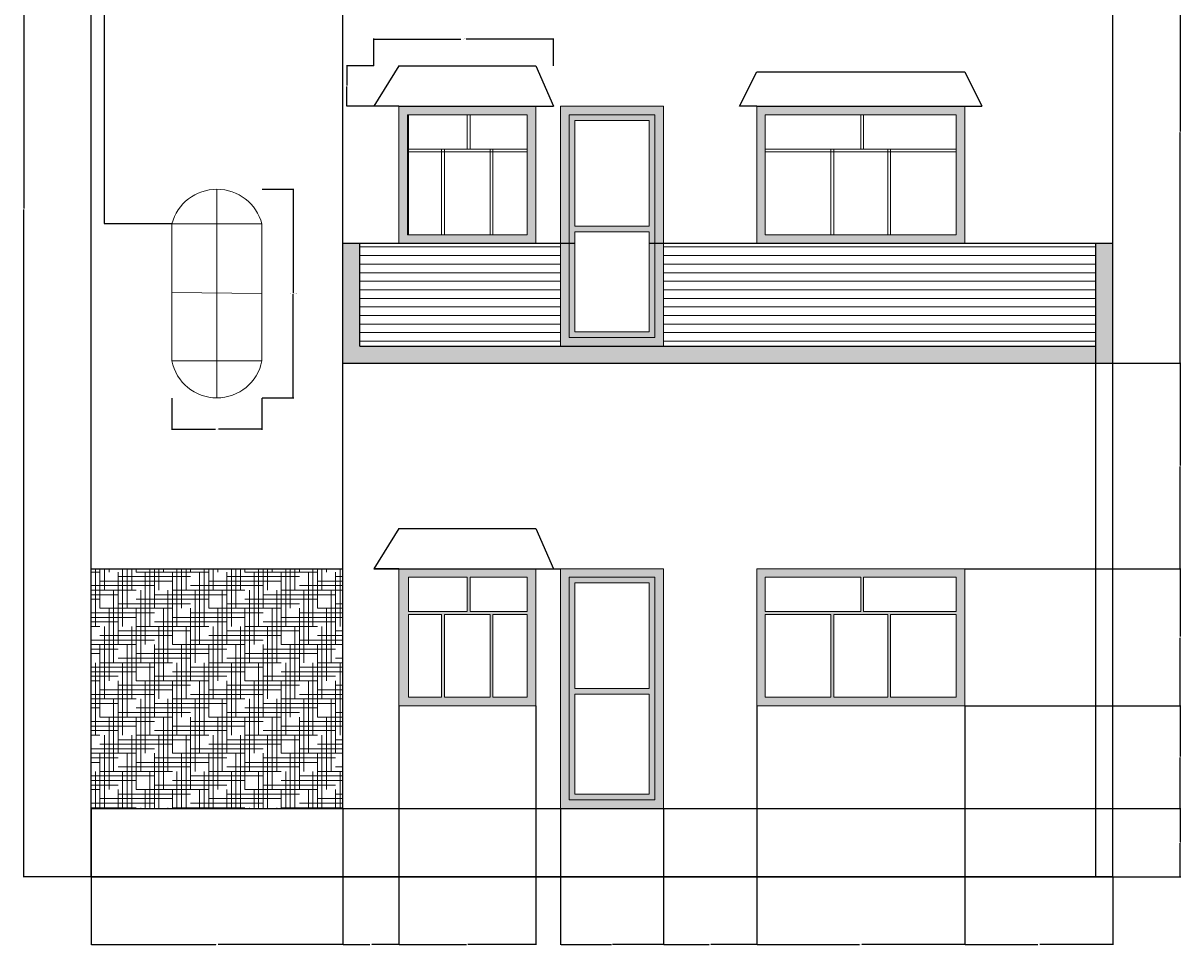
# Model space of a CAD drawing. Units: inches. Extents: x 3504 to 4623, y 2365 to 3357.
# Tile 2 of 5: x 3504 to 3909, y 2841 to 3164. Entities that reach past the tile are written whole.
import ezdxf

# ---------------------------------------------------------------- set-up
doc = ezdxf.new("R2010")
doc.units = ezdxf.units.IN
for name, color, linetype, lineweight in [('A-ANNO-DIMS', 2, 'Continuous', 18), ('A-DOOR', 3, 'Continuous', 18), ('A-ELEV', 7, 'Continuous', 25), ('A-ELEV-PATT', 7, 'Continuous', 13), ('A-FLOR-HRAL', 7, 'Continuous', 25), ('A-FLOR-HRAL-PATT', 252, 'Continuous', 13), ('A-GLAZ', 4, 'Continuous', 18), ('A-ROOF', 7, 'Continuous', 25)]:
    doc.layers.add(name, color=color, linetype=linetype, lineweight=lineweight)
doc.styles.get("Standard").update_dxf_attribs({"font": 'arial.ttf'})
doc.dimstyles.get("Standard").update_dxf_attribs({"dimtxt": 0.18, "dimasz": 0.18, "dimexe": 0.18, "dimexo": 0.0625, "dimgap": 0.09, "dimtad": 0, "dimtih": 1, "dimtoh": 1, "dimdec": 4, "dimzin": 0, "dimdsep": 46, "dimtxsty": 'Standard', "dimcen": 0.09, "dimadec": 0, "dimazin": 0, "dimtfac": 1, "dimtdec": 4, "dimtofl": 0, "dimtmove": 0, "dimatfit": 3, "dimfxl": 1, "dimtolj": 1, "dimtzin": 0, "dimarcsym": 0})

# ---------------------------------------------------------------- blocks, each defined once
blk = doc.blocks.new('WIN-ARCH-END-ELEV')
for p, q in [((15.78, 73.08), (15.78, 0)), ((0, 60.97), (31.56, 60.97)), ((0, 60.97), (0, 12.97)), ((31.56, 12.97), (31.56, 60.97)), ((0, 36.97), (31.56, 36.54)), ((0, 12.97), (31.56, 12.97)), ((0, 12.97), (31.56, 12.97))]:
    blk.add_line(p, q)
for centre, radius, start, end in [((15.78, 56.75), 16.33, 14.9627, 165.0373), ((15.78, 16.08), 16.08, 191.1699, 348.8301)]:
    blk.add_arc(centre, radius, start, end)
blk = doc.blocks.new('WINDOW-HOOD-CAP-48')
for p, q in [((8.73, 14.1), (0, 0)), ((8.73, 14.1), (56.73, 14.1)), ((56.73, 14.1), (62.87, 0))]:
    blk.add_line(p, q)
blk = doc.blocks.new('*D19')
at = {"layer": 'A-ANNO-DIMS', "color": 0, "lineweight": -2, "transparency": 16777216}
for p, q in [((3587.42, 3105.9), (3598.5, 3105.9)), ((3598.32, 3105.72), (3598.32, 3069.54)), ((3598.32, 3032.99), (3598.32, 3069.17)), ((3587.42, 3032.81), (3598.5, 3032.81))]:
    blk.add_line(p, q, dxfattribs=at)
at = {"layer": 'A-ANNO-DIMS', "color": 0, "transparency": 16777216}
for points in [[(3598.29, 3105.72), (3598.35, 3105.72), (3598.32, 3105.9)], [(3598.29, 3032.99), (3598.35, 3032.99), (3598.32, 3032.81)]]:
    blk.add_solid(points, dxfattribs=at)
at = {"layer": 'Defpoints', "color": 0, "transparency": 16777216}
for p in [(3587.36, 3105.9), (3598.32, 3105.9), (3587.36, 3032.81)]:
    blk.add_point(p, dxfattribs=at)
at = {"layer": 'A-ANNO-DIMS', "color": 0, "transparency": 16777216, "insert": (3598.32, 3069.35), "char_height": 0.18, "attachment_point": 5}
blk.add_mtext('\\A1;STAIR WINDOW 73 TYP.', dxfattribs=at)
blk = doc.blocks.new('*D20')
at = {"layer": 'A-ANNO-DIMS', "color": 0, "lineweight": -2, "transparency": 16777216}
for p, q in [((3555.8, 3032.75), (3555.8, 3021.67)), ((3587.36, 3032.75), (3587.36, 3021.67)), ((3555.98, 3021.85), (3571.05, 3021.85)), ((3587.18, 3021.85), (3572.11, 3021.85))]:
    blk.add_line(p, q, dxfattribs=at)
at = {"layer": 'A-ANNO-DIMS', "color": 0, "transparency": 16777216}
for points in [[(3555.98, 3021.88), (3555.98, 3021.82), (3555.8, 3021.85)], [(3587.18, 3021.88), (3587.18, 3021.82), (3587.36, 3021.85)]]:
    blk.add_solid(points, dxfattribs=at)
at = {"layer": 'Defpoints', "color": 0, "transparency": 16777216}
for p in [(3555.8, 3032.81), (3587.36, 3032.81), (3587.36, 3021.85)]:
    blk.add_point(p, dxfattribs=at)
at = {"layer": 'A-ANNO-DIMS', "color": 0, "transparency": 16777216, "insert": (3571.58, 3021.85), "char_height": 0.18, "attachment_point": 5}
blk.add_mtext('\\A1;32 TYP.', dxfattribs=at)
blk = doc.blocks.new('*D21')
at = {"layer": 'A-ANNO-DIMS', "color": 0, "lineweight": -2, "transparency": 16777216}
for p, q in [((3626.58, 3149.15), (3626.58, 3158.69)), ((3626.76, 3158.51), (3657.08, 3158.51)), ((3689.27, 3158.51), (3658.95, 3158.51)), ((3689.45, 3149.15), (3689.45, 3158.69))]:
    blk.add_line(p, q, dxfattribs=at)
at = {"layer": 'A-ANNO-DIMS', "color": 0, "transparency": 16777216}
for points in [[(3626.76, 3158.54), (3626.76, 3158.48), (3626.58, 3158.51)], [(3689.27, 3158.54), (3689.27, 3158.48), (3689.45, 3158.51)]]:
    blk.add_solid(points, dxfattribs=at)
at = {"layer": 'Defpoints', "color": 0, "transparency": 16777216}
for p in [(3689.45, 3158.51), (3626.58, 3149.08), (3689.45, 3149.08)]:
    blk.add_point(p, dxfattribs=at)
at = {"layer": 'A-ANNO-DIMS', "color": 0, "transparency": 16777216, "insert": (3658.01, 3158.51), "char_height": 0.18, "attachment_point": 5}
blk.add_mtext('\\A1;HOOD 63 TYP.', dxfattribs=at)
blk = doc.blocks.new('*D22')
at = {"layer": 'A-ANNO-DIMS', "color": 0, "lineweight": -2, "transparency": 16777216}
for p, q in [((3626.52, 3149.08), (3616.97, 3149.08)), ((3617.15, 3148.9), (3617.15, 3142.21)), ((3617.15, 3135.16), (3617.15, 3141.85)), ((3626.52, 3134.98), (3616.97, 3134.98))]:
    blk.add_line(p, q, dxfattribs=at)
at = {"layer": 'A-ANNO-DIMS', "color": 0, "transparency": 16777216}
for points in [[(3617.12, 3148.9), (3617.18, 3148.9), (3617.15, 3149.08)], [(3617.12, 3135.16), (3617.18, 3135.16), (3617.15, 3134.98)]]:
    blk.add_solid(points, dxfattribs=at)
at = {"layer": 'Defpoints', "color": 0, "transparency": 16777216}
for p in [(3617.15, 3149.08), (3626.58, 3149.08), (3626.58, 3134.98)]:
    blk.add_point(p, dxfattribs=at)
at = {"layer": 'A-ANNO-DIMS', "color": 0, "transparency": 16777216, "insert": (3617.15, 3142.03), "char_height": 0.18, "attachment_point": 5}
blk.add_mtext('\\A1;14 TYP.', dxfattribs=at)
blk = doc.blocks.new('*D48')
at = {"layer": 'A-ANNO-DIMS', "color": 0, "lineweight": -2, "transparency": 16777216}
for p, q in [((3527.5, 2888.92), (3527.5, 2841.2)), ((3615.67, 2888.92), (3615.67, 2841.2)), ((3527.68, 2841.38), (3571.19, 2841.38)), ((3615.49, 2841.38), (3571.98, 2841.38))]:
    blk.add_line(p, q, dxfattribs=at)
at = {"layer": 'A-ANNO-DIMS', "color": 0, "transparency": 16777216}
for points in [[(3527.68, 2841.41), (3527.68, 2841.35), (3527.5, 2841.38)], [(3615.49, 2841.41), (3615.49, 2841.35), (3615.67, 2841.38)]]:
    blk.add_solid(points, dxfattribs=at)
at = {"layer": 'Defpoints', "color": 0, "transparency": 16777216}
for p in [(3527.5, 2888.98), (3615.67, 2888.98), (3615.67, 2841.38)]:
    blk.add_point(p, dxfattribs=at)
at = {"layer": 'A-ANNO-DIMS', "color": 0, "transparency": 16777216, "insert": (3571.58, 2841.38), "char_height": 0.18, "attachment_point": 5}
blk.add_mtext('\\A1;88.17', dxfattribs=at)
blk = doc.blocks.new('*D49')
at = {"layer": 'A-ANNO-DIMS', "color": 0, "lineweight": -2, "transparency": 16777216}
for p, q in [((3635.31, 2924.92), (3635.31, 2841.2)), ((3615.67, 2888.92), (3615.67, 2841.2)), ((3615.85, 2841.38), (3625.1, 2841.38)), ((3635.13, 2841.38), (3625.87, 2841.38))]:
    blk.add_line(p, q, dxfattribs=at)
at = {"layer": 'A-ANNO-DIMS', "color": 0, "transparency": 16777216}
for points in [[(3615.85, 2841.41), (3615.85, 2841.35), (3615.67, 2841.38)], [(3635.13, 2841.41), (3635.13, 2841.35), (3635.31, 2841.38)]]:
    blk.add_solid(points, dxfattribs=at)
at = {"layer": 'Defpoints', "color": 0, "transparency": 16777216}
for p in [(3635.31, 2924.98), (3615.67, 2888.98), (3635.31, 2841.38)]:
    blk.add_point(p, dxfattribs=at)
at = {"layer": 'A-ANNO-DIMS', "color": 0, "transparency": 16777216, "insert": (3625.49, 2841.38), "char_height": 0.18, "attachment_point": 5}
blk.add_mtext('\\A1;19.64', dxfattribs=at)
blk = doc.blocks.new('*D50')
at = {"layer": 'A-ANNO-DIMS', "color": 0, "lineweight": -2, "transparency": 16777216}
for p, q in [((3635.31, 2924.92), (3635.31, 2841.2)), ((3683.31, 2924.92), (3683.31, 2841.2)), ((3635.49, 2841.38), (3659.08, 2841.38)), ((3683.13, 2841.38), (3659.53, 2841.38))]:
    blk.add_line(p, q, dxfattribs=at)
at = {"layer": 'A-ANNO-DIMS', "color": 0, "transparency": 16777216}
for points in [[(3635.49, 2841.41), (3635.49, 2841.35), (3635.31, 2841.38)], [(3683.13, 2841.41), (3683.13, 2841.35), (3683.31, 2841.38)]]:
    blk.add_solid(points, dxfattribs=at)
at = {"layer": 'Defpoints', "color": 0, "transparency": 16777216}
for p in [(3635.31, 2924.98), (3683.31, 2924.98), (3683.31, 2841.38)]:
    blk.add_point(p, dxfattribs=at)
at = {"layer": 'A-ANNO-DIMS', "color": 0, "transparency": 16777216, "insert": (3659.31, 2841.38), "char_height": 0.18, "attachment_point": 5}
blk.add_mtext('\\A1;48', dxfattribs=at)
blk = doc.blocks.new('*D51')
at = {"layer": 'A-ANNO-DIMS', "color": 0, "lineweight": -2, "transparency": 16777216}
for p, q in [((3692, 2888.92), (3692, 2841.2)), ((3728, 2888.92), (3728, 2841.2)), ((3692.18, 2841.38), (3709.78, 2841.38)), ((3727.82, 2841.38), (3710.22, 2841.38))]:
    blk.add_line(p, q, dxfattribs=at)
at = {"layer": 'A-ANNO-DIMS', "color": 0, "transparency": 16777216}
for points in [[(3692.18, 2841.41), (3692.18, 2841.35), (3692, 2841.38)], [(3727.82, 2841.41), (3727.82, 2841.35), (3728, 2841.38)]]:
    blk.add_solid(points, dxfattribs=at)
at = {"layer": 'Defpoints', "color": 0, "transparency": 16777216}
for p in [(3692, 2888.98), (3728, 2888.98), (3728, 2841.38)]:
    blk.add_point(p, dxfattribs=at)
at = {"layer": 'A-ANNO-DIMS', "color": 0, "transparency": 16777216, "insert": (3710, 2841.38), "char_height": 0.18, "attachment_point": 5}
blk.add_mtext('\\A1;36', dxfattribs=at)
blk = doc.blocks.new('*D52')
at = {"layer": 'A-ANNO-DIMS', "color": 0, "lineweight": -2, "transparency": 16777216}
for p, q in [((3760.69, 2924.92), (3760.69, 2841.2)), ((3728, 2888.92), (3728, 2841.2)), ((3728.18, 2841.38), (3744.02, 2841.38)), ((3760.51, 2841.38), (3744.67, 2841.38))]:
    blk.add_line(p, q, dxfattribs=at)
at = {"layer": 'A-ANNO-DIMS', "color": 0, "transparency": 16777216}
for points in [[(3728.18, 2841.41), (3728.18, 2841.35), (3728, 2841.38)], [(3760.51, 2841.41), (3760.51, 2841.35), (3760.69, 2841.38)]]:
    blk.add_solid(points, dxfattribs=at)
at = {"layer": 'Defpoints', "color": 0, "transparency": 16777216}
for p in [(3760.69, 2924.98), (3728, 2888.98), (3760.69, 2841.38)]:
    blk.add_point(p, dxfattribs=at)
at = {"layer": 'A-ANNO-DIMS', "color": 0, "transparency": 16777216, "insert": (3744.35, 2841.38), "char_height": 0.18, "attachment_point": 5}
blk.add_mtext('\\A1;32.7', dxfattribs=at)
blk = doc.blocks.new('*D53')
at = {"layer": 'A-ANNO-DIMS', "color": 0, "lineweight": -2, "transparency": 16777216}
for p, q in [((3760.69, 2924.92), (3760.69, 2841.2)), ((3833.61, 2924.92), (3833.61, 2841.2)), ((3760.87, 2841.38), (3796.76, 2841.38)), ((3833.43, 2841.38), (3797.55, 2841.38))]:
    blk.add_line(p, q, dxfattribs=at)
at = {"layer": 'A-ANNO-DIMS', "color": 0, "transparency": 16777216}
for points in [[(3760.87, 2841.41), (3760.87, 2841.35), (3760.69, 2841.38)], [(3833.43, 2841.41), (3833.43, 2841.35), (3833.61, 2841.38)]]:
    blk.add_solid(points, dxfattribs=at)
at = {"layer": 'Defpoints', "color": 0, "transparency": 16777216}
for p in [(3760.69, 2924.98), (3833.61, 2924.98), (3833.61, 2841.38)]:
    blk.add_point(p, dxfattribs=at)
at = {"layer": 'A-ANNO-DIMS', "color": 0, "transparency": 16777216, "insert": (3797.15, 2841.38), "char_height": 0.18, "attachment_point": 5}
blk.add_mtext('\\A1;72.92', dxfattribs=at)
blk = doc.blocks.new('*D54')
at = {"layer": 'A-ANNO-DIMS', "color": 0, "lineweight": -2, "transparency": 16777216}
for p, q in [((3833.61, 2924.92), (3833.61, 2841.2)), ((3885.5, 2864.92), (3885.5, 2841.2)), ((3833.79, 2841.38), (3859.16, 2841.38)), ((3885.32, 2841.38), (3859.95, 2841.38))]:
    blk.add_line(p, q, dxfattribs=at)
at = {"layer": 'A-ANNO-DIMS', "color": 0, "transparency": 16777216}
for points in [[(3833.79, 2841.41), (3833.79, 2841.35), (3833.61, 2841.38)], [(3885.32, 2841.41), (3885.32, 2841.35), (3885.5, 2841.38)]]:
    blk.add_solid(points, dxfattribs=at)
at = {"layer": 'Defpoints', "color": 0, "transparency": 16777216}
for p in [(3833.61, 2924.98), (3885.5, 2864.98), (3885.5, 2841.38)]:
    blk.add_point(p, dxfattribs=at)
at = {"layer": 'A-ANNO-DIMS', "color": 0, "transparency": 16777216, "insert": (3859.55, 2841.38), "char_height": 0.18, "attachment_point": 5}
blk.add_mtext('\\A1;51.88', dxfattribs=at)
blk = doc.blocks.new('*D55')
at = {"layer": 'A-ANNO-DIMS', "color": 0, "lineweight": -2, "transparency": 16777216}
for p, q in [((3885.56, 2888.98), (3909.28, 2888.98)), ((3909.1, 2888.8), (3909.1, 2877.16)), ((3909.1, 2865.16), (3909.1, 2876.8)), ((3885.56, 2864.98), (3909.28, 2864.98))]:
    blk.add_line(p, q, dxfattribs=at)
at = {"layer": 'A-ANNO-DIMS', "color": 0, "transparency": 16777216}
for points in [[(3909.07, 2888.8), (3909.13, 2888.8), (3909.1, 2888.98)], [(3909.07, 2865.16), (3909.13, 2865.16), (3909.1, 2864.98)]]:
    blk.add_solid(points, dxfattribs=at)
at = {"layer": 'Defpoints', "color": 0, "transparency": 16777216}
for p in [(3885.5, 2888.98), (3909.1, 2888.98), (3885.5, 2864.98)]:
    blk.add_point(p, dxfattribs=at)
at = {"layer": 'A-ANNO-DIMS', "color": 0, "transparency": 16777216, "insert": (3909.1, 2876.98), "char_height": 0.18, "attachment_point": 5}
blk.add_mtext('\\A1;24', dxfattribs=at)
blk = doc.blocks.new('*D56')
at = {"layer": 'A-ANNO-DIMS', "color": 0, "lineweight": -2, "transparency": 16777216}
for p, q in [((3833.68, 2924.98), (3909.28, 2924.98)), ((3909.1, 2924.8), (3909.1, 2907.17)), ((3909.1, 2889.16), (3909.1, 2906.8)), ((3885.56, 2888.98), (3909.28, 2888.98))]:
    blk.add_line(p, q, dxfattribs=at)
at = {"layer": 'A-ANNO-DIMS', "color": 0, "transparency": 16777216}
for points in [[(3909.07, 2924.8), (3909.13, 2924.8), (3909.1, 2924.98)], [(3909.07, 2889.16), (3909.13, 2889.16), (3909.1, 2888.98)]]:
    blk.add_solid(points, dxfattribs=at)
at = {"layer": 'Defpoints', "color": 0, "transparency": 16777216}
for p in [(3833.61, 2924.98), (3909.1, 2924.98), (3885.5, 2888.98)]:
    blk.add_point(p, dxfattribs=at)
at = {"layer": 'A-ANNO-DIMS', "color": 0, "transparency": 16777216, "insert": (3909.1, 2906.98), "char_height": 0.18, "attachment_point": 5}
blk.add_mtext('\\A1;36', dxfattribs=at)
blk = doc.blocks.new('*D57')
at = {"layer": 'A-ANNO-DIMS', "color": 0, "lineweight": -2, "transparency": 16777216}
for p, q in [((3833.68, 2972.98), (3909.28, 2972.98)), ((3909.1, 2972.8), (3909.1, 2949.17)), ((3909.1, 2925.16), (3909.1, 2948.8)), ((3833.68, 2924.98), (3909.28, 2924.98))]:
    blk.add_line(p, q, dxfattribs=at)
at = {"layer": 'A-ANNO-DIMS', "color": 0, "transparency": 16777216}
for points in [[(3909.07, 2972.8), (3909.13, 2972.8), (3909.1, 2972.98)], [(3909.07, 2925.16), (3909.13, 2925.16), (3909.1, 2924.98)]]:
    blk.add_solid(points, dxfattribs=at)
at = {"layer": 'Defpoints', "color": 0, "transparency": 16777216}
for p in [(3833.61, 2972.98), (3909.1, 2972.98), (3833.61, 2924.98)]:
    blk.add_point(p, dxfattribs=at)
at = {"layer": 'A-ANNO-DIMS', "color": 0, "transparency": 16777216, "insert": (3909.1, 2948.98), "char_height": 0.18, "attachment_point": 5}
blk.add_mtext('\\A1;48', dxfattribs=at)
blk = doc.blocks.new('*D58')
at = {"layer": 'A-ANNO-DIMS', "color": 0, "lineweight": -2, "transparency": 16777216}
for p, q in [((3885.56, 3044.98), (3909.28, 3044.98)), ((3909.1, 3044.8), (3909.1, 3009.16)), ((3909.1, 2973.16), (3909.1, 3008.8)), ((3833.68, 2972.98), (3909.28, 2972.98))]:
    blk.add_line(p, q, dxfattribs=at)
at = {"layer": 'A-ANNO-DIMS', "color": 0, "transparency": 16777216}
for points in [[(3909.07, 3044.8), (3909.13, 3044.8), (3909.1, 3044.98)], [(3909.07, 2973.16), (3909.13, 2973.16), (3909.1, 2972.98)]]:
    blk.add_solid(points, dxfattribs=at)
at = {"layer": 'Defpoints', "color": 0, "transparency": 16777216}
for p in [(3885.5, 3044.98), (3909.1, 3044.98), (3833.61, 2972.98)]:
    blk.add_point(p, dxfattribs=at)
at = {"layer": 'A-ANNO-DIMS', "color": 0, "transparency": 16777216, "insert": (3909.1, 3008.98), "char_height": 0.18, "attachment_point": 5}
blk.add_mtext('\\A1;72', dxfattribs=at)
blk = doc.blocks.new('*D59')
at = {"layer": 'A-ANNO-DIMS', "color": 0, "lineweight": -2, "transparency": 16777216}
for p, q in [((3885.56, 3206.98), (3909.28, 3206.98)), ((3909.1, 3206.8), (3909.1, 3126.17)), ((3909.1, 3045.16), (3909.1, 3125.8)), ((3885.56, 3044.98), (3909.28, 3044.98))]:
    blk.add_line(p, q, dxfattribs=at)
at = {"layer": 'A-ANNO-DIMS', "color": 0, "transparency": 16777216}
for points in [[(3909.07, 3206.8), (3909.13, 3206.8), (3909.1, 3206.98)], [(3909.07, 3045.16), (3909.13, 3045.16), (3909.1, 3044.98)]]:
    blk.add_solid(points, dxfattribs=at)
at = {"layer": 'Defpoints', "color": 0, "transparency": 16777216}
for p in [(3885.5, 3206.98), (3909.1, 3206.98), (3885.5, 3044.98)]:
    blk.add_point(p, dxfattribs=at)
at = {"layer": 'A-ANNO-DIMS', "color": 0, "transparency": 16777216, "insert": (3909.1, 3125.98), "char_height": 0.18, "attachment_point": 5}
blk.add_mtext('\\A1;162', dxfattribs=at)
blk = doc.blocks.new('*D61')
at = {"layer": 'A-ANNO-DIMS', "color": 0, "lineweight": -2, "transparency": 16777216}
for p, q in [((3555.74, 3260.98), (3532.02, 3260.98)), ((3532.2, 3260.8), (3532.2, 3177.56)), ((3532.2, 3093.96), (3532.2, 3177.2)), ((3555.74, 3093.78), (3532.02, 3093.78))]:
    blk.add_line(p, q, dxfattribs=at)
at = {"layer": 'A-ANNO-DIMS', "color": 0, "transparency": 16777216}
for points in [[(3532.17, 3260.8), (3532.23, 3260.8), (3532.2, 3260.98)], [(3532.17, 3093.96), (3532.23, 3093.96), (3532.2, 3093.78)]]:
    blk.add_solid(points, dxfattribs=at)
at = {"layer": 'Defpoints', "color": 0, "transparency": 16777216}
for p in [(3532.2, 3260.98), (3555.8, 3260.98), (3555.8, 3093.78)]:
    blk.add_point(p, dxfattribs=at)
at = {"layer": 'A-ANNO-DIMS', "color": 0, "transparency": 16777216, "insert": (3532.2, 3177.38), "char_height": 0.18, "attachment_point": 5}
blk.add_mtext('\\A1;167.2', dxfattribs=at)
blk = doc.blocks.new('*D63')
at = {"layer": 'A-ANNO-DIMS', "color": 0, "lineweight": -2, "transparency": 16777216}
for p, q in [((3527.43, 3332.98), (3503.72, 3332.98)), ((3503.9, 3332.8), (3503.9, 3099.17)), ((3503.9, 2865.16), (3503.9, 3098.8)), ((3527.43, 2864.98), (3503.72, 2864.98))]:
    blk.add_line(p, q, dxfattribs=at)
at = {"layer": 'A-ANNO-DIMS', "color": 0, "transparency": 16777216}
for points in [[(3503.87, 3332.8), (3503.93, 3332.8), (3503.9, 3332.98)], [(3503.87, 2865.16), (3503.93, 2865.16), (3503.9, 2864.98)]]:
    blk.add_solid(points, dxfattribs=at)
at = {"layer": 'Defpoints', "color": 0, "transparency": 16777216}
for p in [(3503.9, 3332.98), (3527.5, 3332.98), (3527.5, 2864.98)]:
    blk.add_point(p, dxfattribs=at)
at = {"layer": 'A-ANNO-DIMS', "color": 0, "transparency": 16777216, "insert": (3503.9, 3098.98), "char_height": 0.18, "attachment_point": 5}
blk.add_mtext('\\A1;468', dxfattribs=at)

msp = doc.modelspace()

# ---------------------------------------------------------------- hatches: boundary and pattern name
at = {"layer": 'A-ELEV-PATT'}
h = msp.add_hatch(color=256, dxfattribs=at)
h.dxf.hatch_style = 1
h.paths.add_polyline_path([(3683.3055, 3134.9837), (3635.3055, 3134.9837), (3635.3055, 3086.9837), (3683.3055, 3086.9837)])
h.paths.add_polyline_path([(3680.3055, 3131.9837), (3680.3055, 3089.9837), (3638.3055, 3089.9837), (3638.3055, 3131.9837)], flags=16)
h.paths.add_polyline_path([(3668.3055, 3119.9837), (3668.3055, 3118.9837), (3638.6868, 3118.9837), (3638.6868, 3119.9837)], flags=0)
h.paths.add_polyline_path([(3651.3055, 3118.9837), (3650.3055, 3118.9837), (3650.3055, 3089.9837), (3651.3055, 3089.9837)], flags=0)
h.paths.add_polyline_path([(3668.3055, 3118.9837), (3667.3055, 3118.9837), (3667.3055, 3089.9837), (3668.3055, 3089.9837)], flags=0)
h.paths.add_polyline_path([(3724.9963, 3131.9837), (3694.9963, 3131.9837), (3694.9963, 3053.9837), (3724.9963, 3053.9837)], flags=0)
h.paths.add_polyline_path([(3696.9963, 3129.9837), (3722.9963, 3129.9837), (3722.9963, 3092.9837), (3696.9963, 3092.9837)], flags=0)
h.paths.add_polyline_path([(3696.9963, 3090.9837), (3722.9963, 3090.9837), (3722.9963, 3055.9837), (3696.9963, 3055.9837)], flags=0)
h.paths.add_polyline_path([(3727.9963, 3134.9837), (3691.9963, 3134.9837), (3691.9963, 3050.9837), (3727.9963, 3050.9837)])
h.paths.add_polyline_path([(3694.9963, 3131.9837), (3724.9963, 3131.9837), (3724.9963, 3053.9837), (3694.9963, 3053.9837)], flags=16)
h.paths.add_polyline_path([(3833.6131, 3134.9837), (3760.6941, 3134.9837), (3760.6941, 3086.9837), (3833.6131, 3086.9837)])
h.paths.add_polyline_path([(3763.6941, 3131.9837), (3830.6131, 3131.9837), (3830.6131, 3089.9837), (3763.6941, 3089.9837)], flags=16)
h.paths.add_polyline_path([(3807.6131, 3119.9837), (3807.6131, 3118.9837), (3786.6941, 3118.9837), (3786.6941, 3119.9837)], flags=0)
h.paths.add_polyline_path([(3680.3055, 3119.9837), (3668.3055, 3119.9837), (3668.3055, 3118.9837), (3680.3055, 3118.9837)], flags=0)
h.paths.add_polyline_path([(3660.3055, 3131.9837), (3659.3055, 3131.9837), (3659.3055, 3119.9837), (3660.3055, 3119.9837)], flags=0)
h.paths.add_polyline_path([(3787.6941, 3118.9837), (3786.6941, 3118.9837), (3786.6941, 3089.9837), (3787.6941, 3089.9837)], flags=0)
h.paths.add_polyline_path([(3807.6131, 3118.9837), (3806.6131, 3118.9837), (3806.6131, 3089.9837), (3807.6131, 3089.9837)], flags=0)
h.paths.add_polyline_path([(3786.6941, 3119.9837), (3763.6941, 3119.9837), (3763.6941, 3118.9837), (3786.6941, 3118.9837)], flags=0)
h.paths.add_polyline_path([(3787.6941, 3119.9837), (3786.6941, 3119.9837), (3786.6941, 3118.9837), (3787.6941, 3118.9837)], flags=0)
h.paths.add_polyline_path([(3807.6131, 3119.9837), (3806.6131, 3119.9837), (3806.6131, 3118.9837), (3807.6131, 3118.9837)], flags=0)
h.paths.add_polyline_path([(3798.1536, 3131.9837), (3797.1536, 3131.9837), (3797.1536, 3119.9837), (3798.1536, 3119.9837)], flags=0)
h.paths.add_polyline_path([(3830.6131, 3119.9837), (3807.6131, 3119.9837), (3807.6131, 3118.9837), (3830.6131, 3118.9837)], flags=0)
h = msp.add_hatch(color=256, dxfattribs=at)
h.dxf.hatch_style = 1
h.paths.add_polyline_path([(3724.9963, 3131.9837), (3694.9963, 3131.9837), (3694.9963, 3053.9837), (3724.9963, 3053.9837)])
h.paths.add_polyline_path([(3696.9963, 3092.9837), (3696.9963, 3129.9837), (3722.9963, 3129.9837), (3722.9963, 3092.9837)], flags=16)
h.paths.add_polyline_path([(3722.9963, 3090.9837), (3722.9963, 3055.9837), (3696.9963, 3055.9837), (3696.9963, 3090.9837)], flags=16)
h = msp.add_hatch(color=256, dxfattribs=at)
h.dxf.hatch_style = 1
h.paths.add_polyline_path([(3885.4963, 3086.9837), (3879.4963, 3086.9837), (3879.4963, 3050.9837), (3621.6665, 3050.9837), (3621.6665, 3086.9837), (3615.6665, 3086.9837), (3615.6665, 3044.9837), (3885.4963, 3044.9837)])
h = msp.add_hatch(dxfattribs=at)
h.set_pattern_fill('HOUND', color=256)
h.paths.add_polyline_path([(3527.4963, 2972.9837), (3527.4963, 2888.9837), (3615.6665, 2888.9837), (3615.6665, 2972.9837)])
h = msp.add_hatch(color=256, dxfattribs=at)
h.dxf.hatch_style = 1
h.paths.add_polyline_path([(3683.3055, 2972.9837), (3635.3055, 2972.9837), (3635.3055, 2924.9837), (3683.3055, 2924.9837)])
h.paths.add_polyline_path([(3638.6868, 2956.9837), (3650.3055, 2956.9837), (3650.3055, 2927.9837), (3638.6868, 2927.9837)], flags=16)
h.paths.add_polyline_path([(3651.3055, 2956.9837), (3667.3055, 2956.9837), (3667.3055, 2927.9837), (3651.3055, 2927.9837)], flags=16)
h.paths.add_polyline_path([(3638.6868, 2957.9837), (3638.6868, 2969.9837), (3659.3055, 2969.9837), (3659.3055, 2957.9837)], flags=16)
h.paths.add_polyline_path([(3660.3055, 2957.9837), (3660.3055, 2969.9837), (3680.3055, 2969.9837), (3680.3055, 2957.9837)], flags=16)
h.paths.add_polyline_path([(3668.3055, 2956.9837), (3680.3055, 2956.9837), (3680.3055, 2927.9837), (3668.3055, 2927.9837)], flags=16)
h = msp.add_hatch(color=256, dxfattribs=at)
h.dxf.hatch_style = 1
h.paths.add_polyline_path([(3724.9963, 2969.9837), (3694.9963, 2969.9837), (3694.9963, 2891.9837), (3724.9963, 2891.9837)], flags=0)
h.paths.add_polyline_path([(3696.9963, 2967.9837), (3722.9963, 2967.9837), (3722.9963, 2930.9837), (3696.9963, 2930.9837)], flags=0)
h.paths.add_polyline_path([(3696.9963, 2928.9837), (3722.9963, 2928.9837), (3722.9963, 2893.9837), (3696.9963, 2893.9837)], flags=0)
h.paths.add_polyline_path([(3727.9963, 2972.9837), (3691.9963, 2972.9837), (3691.9963, 2888.9837), (3727.9963, 2888.9837)])
h.paths.add_polyline_path([(3694.9963, 2969.9837), (3724.9963, 2969.9837), (3724.9963, 2891.9837), (3694.9963, 2891.9837)], flags=16)
h = msp.add_hatch(color=256, dxfattribs=at)
h.dxf.hatch_style = 1
h.paths.add_polyline_path([(3724.9963, 2969.9837), (3694.9963, 2969.9837), (3694.9963, 2891.9837), (3724.9963, 2891.9837)])
h.paths.add_polyline_path([(3696.9963, 2930.9837), (3696.9963, 2967.9837), (3722.9963, 2967.9837), (3722.9963, 2930.9837)], flags=16)
h.paths.add_polyline_path([(3722.9963, 2928.9837), (3722.9963, 2893.9837), (3696.9963, 2893.9837), (3696.9963, 2928.9837)], flags=16)
h = msp.add_hatch(color=256, dxfattribs=at)
h.dxf.hatch_style = 1
h.paths.add_polyline_path([(3833.6131, 2972.9837), (3760.6941, 2972.9837), (3760.6941, 2924.9837), (3833.6131, 2924.9837)])
h.paths.add_polyline_path([(3797.1536, 2957.9837), (3763.6941, 2957.9837), (3763.6941, 2969.9837), (3797.1536, 2969.9837)], flags=16)
h.paths.add_polyline_path([(3798.1536, 2969.9837), (3830.6131, 2969.9837), (3830.6131, 2957.9837), (3798.1536, 2957.9837)], flags=16)
h.paths.add_polyline_path([(3806.6131, 2956.9837), (3806.6131, 2927.9837), (3787.6941, 2927.9837), (3787.6941, 2956.9837)], flags=16)
h.paths.add_polyline_path([(3807.6131, 2956.9837), (3830.6131, 2956.9837), (3830.6131, 2927.9837), (3807.6131, 2927.9837)], flags=16)
h.paths.add_polyline_path([(3786.6941, 2956.9837), (3786.6941, 2927.9837), (3763.6941, 2927.9837), (3763.6941, 2956.9837)], flags=16)
at = {"layer": 'A-FLOR-HRAL-PATT'}
h = msp.add_hatch(dxfattribs=at)
h.set_pattern_fill('ANSI31', color=256, scale=0.944475, angle=-45, style=0)
h.paths.add_polyline_path([(3621.6665, 3050.9837), (3691.9963, 3050.9837), (3691.9963, 3086.9837), (3621.6665, 3086.9837)])
h = msp.add_hatch(dxfattribs=at)
h.set_pattern_fill('ANSI31', color=256, scale=0.944475, angle=-45, style=0)
h.paths.add_polyline_path([(3727.9963, 3050.9837), (3879.4963, 3050.9837), (3879.4963, 3086.9837), (3727.9963, 3086.9837)])

# ---------------------------------------------------------------- linework, layer by layer
at = {"layer": 'A-DOOR'}
for p, q in [((3691.9963, 3086.9837), (3691.9963, 3134.9837)), ((3691.9963, 3134.9837), (3727.9963, 3134.9837)), ((3691.9963, 3050.9837), (3691.9963, 3134.9837)), ((3727.9963, 3086.9837), (3727.9963, 3134.9837)), ((3727.9963, 3050.9837), (3727.9963, 3134.9837)), ((3709.9963, 3092.9837), (3696.9963, 3092.9837)), ((3696.9963, 3092.9837), (3722.9963, 3092.9837)), ((3696.9963, 3090.9837), (3722.9963, 3090.9837)), ((3691.9963, 2888.9837), (3691.9963, 2972.9837)), ((3727.9963, 2888.9837), (3727.9963, 2972.9837)), ((3709.9963, 2930.9837), (3696.9963, 2930.9837)), ((3696.9963, 2930.9837), (3722.9963, 2930.9837)), ((3696.9963, 2928.9837), (3722.9963, 2928.9837))]:
    msp.add_line(p, q, dxfattribs=at)
for points in [[(3691.9963, 3050.9837), (3727.9963, 3050.9837), (3727.9963, 3134.9837), (3691.9963, 3134.9837)], [(3691.9963, 3050.9837), (3727.9963, 3050.9837), (3727.9963, 3134.9837), (3691.9963, 3134.9837)], [(3694.9963, 3053.9837), (3724.9963, 3053.9837), (3724.9963, 3131.9837), (3694.9963, 3131.9837)], [(3691.9963, 2888.9837), (3727.9963, 2888.9837), (3727.9963, 2972.9837), (3691.9963, 2972.9837)], [(3694.9963, 2891.9837), (3724.9963, 2891.9837), (3724.9963, 2969.9837), (3694.9963, 2969.9837)]]:
    msp.add_lwpolyline(points, close=True, dxfattribs=at)
for points in [[(3722.9963, 3092.9837), (3722.9963, 3129.9837), (3696.9963, 3129.9837), (3696.9963, 3092.9837)], [(3696.9963, 3090.9837), (3696.9963, 3055.9837), (3722.9963, 3055.9837), (3722.9963, 3090.9837)], [(3722.9963, 2930.9837), (3722.9963, 2967.9837), (3696.9963, 2967.9837), (3696.9963, 2930.9837)], [(3696.9963, 2928.9837), (3696.9963, 2893.9837), (3722.9963, 2893.9837), (3722.9963, 2928.9837)]]:
    msp.add_lwpolyline(points, dxfattribs=at)
at = {"layer": 'A-ELEV'}
for p, q in [((3527.4963, 2864.9837), (3527.4963, 3332.9837)), ((3615.6665, 2888.9837), (3615.6665, 3332.9837)), ((3885.4963, 2864.9837), (3885.4963, 3254.9837)), ((3879.4963, 2864.9837), (3879.4963, 3086.9837)), ((3527.4963, 2972.9837), (3615.6665, 2972.9837)), ((3527.4963, 2888.9837), (3691.9963, 2888.9837)), ((3691.9963, 2888.9837), (3885.4963, 2888.9837)), ((3527.4963, 2864.9837), (3885.4963, 2864.9837)), ((3885.4963, 2864.9837), (3527.4963, 2864.9837)), ((3885.4963, 2864.9837), (3527.4963, 2864.9837))]:
    msp.add_line(p, q, dxfattribs=at)
at = {"layer": 'A-FLOR-HRAL'}
for p, q in [((3615.6665, 3086.9837), (3696.9963, 3086.9837)), ((3621.6665, 3050.9837), (3621.6665, 3086.9837)), ((3722.9963, 3086.9837), (3885.4963, 3086.9837)), ((3879.4963, 3050.9837), (3879.4963, 3086.9837)), ((3621.6665, 3050.9837), (3879.4963, 3050.9837)), ((3615.6665, 3044.9837), (3885.4963, 3044.9837))]:
    msp.add_line(p, q, dxfattribs=at)
at = {"layer": 'A-GLAZ'}
for p, q in [((3635.3055, 3086.9837), (3635.3055, 3134.9837)), ((3635.3055, 3134.9837), (3683.3055, 3134.9837)), ((3635.3055, 3086.9837), (3635.3055, 3134.9837)), ((3635.3055, 3134.9837), (3683.3055, 3134.9837)), ((3638.3055, 3089.9837), (3638.3055, 3131.9837)), ((3638.3055, 3131.9837), (3680.3055, 3131.9837)), ((3638.6868, 3089.9837), (3638.6868, 3131.9837)), ((3659.3055, 3119.9837), (3659.3055, 3131.9837)), ((3660.3055, 3119.9837), (3660.3055, 3131.9837)), ((3680.3055, 3089.9837), (3680.3055, 3131.9837)), ((3683.3055, 3086.9837), (3683.3055, 3134.9837)), ((3683.3055, 3086.9837), (3683.3055, 3134.9837)), ((3760.6941, 3086.9837), (3760.6941, 3134.9837)), ((3760.6941, 3134.9837), (3833.6131, 3134.9837)), ((3760.6941, 3086.9837), (3760.6941, 3134.9837)), ((3833.6131, 3134.9837), (3760.6941, 3134.9837)), ((3760.6941, 3134.9837), (3760.6941, 3086.9837)), ((3830.6131, 3131.9837), (3763.6941, 3131.9837)), ((3763.6941, 3131.9837), (3763.6941, 3089.9837)), ((3797.1536, 3119.9837), (3797.1536, 3131.9837)), ((3798.1536, 3119.9837), (3798.1536, 3131.9837)), ((3830.6131, 3089.9837), (3830.6131, 3131.9837)), ((3833.6131, 3086.9837), (3833.6131, 3134.9837)), ((3833.6131, 3086.9837), (3833.6131, 3134.9837)), ((3833.6131, 3086.9837), (3833.6131, 3134.9837)), ((3638.3055, 3119.9837), (3680.3055, 3119.9837)), ((3650.3055, 3089.9837), (3650.3055, 3119.9837)), ((3651.3055, 3089.9837), (3651.3055, 3119.9837)), ((3667.3055, 3089.9837), (3667.3055, 3119.9837)), ((3668.3055, 3089.9837), (3668.3055, 3119.9837)), ((3830.6131, 3119.9837), (3763.6941, 3119.9837)), ((3786.6941, 3119.9837), (3786.6941, 3089.9837)), ((3787.6941, 3119.9837), (3787.6941, 3089.9837)), ((3806.6131, 3089.9837), (3806.6131, 3119.9837)), ((3807.6131, 3089.9837), (3807.6131, 3119.9837)), ((3638.3055, 3118.9837), (3680.3055, 3118.9837)), ((3830.6131, 3118.9837), (3763.6941, 3118.9837)), ((3635.3055, 3086.9837), (3683.3055, 3086.9837)), ((3635.3055, 3086.9837), (3683.3055, 3086.9837)), ((3638.3055, 3089.9837), (3680.3055, 3089.9837)), ((3760.6941, 3086.9837), (3833.6131, 3086.9837)), ((3760.6941, 3086.9837), (3833.6131, 3086.9837)), ((3760.6941, 3086.9837), (3833.6131, 3086.9837)), ((3833.6131, 3086.9837), (3760.6941, 3086.9837)), ((3760.6941, 3086.9837), (3760.6941, 3086.9837)), ((3760.6941, 3086.9837), (3833.6131, 3086.9837)), ((3763.6941, 3089.9837), (3830.6131, 3089.9837)), ((3833.6131, 3086.9837), (3833.6131, 3086.9837)), ((3635.3055, 2972.9837), (3683.3055, 2972.9837)), ((3635.3055, 2924.9837), (3635.3055, 2972.9837)), ((3638.6868, 2969.9837), (3659.3055, 2969.9837)), ((3638.6868, 2957.9837), (3638.6868, 2969.9837)), ((3659.3055, 2957.9837), (3659.3055, 2969.9837)), ((3660.3055, 2957.9837), (3660.3055, 2969.9837)), ((3660.3055, 2969.9837), (3680.3055, 2969.9837)), ((3680.3055, 2957.9837), (3680.3055, 2969.9837)), ((3683.3055, 2924.9837), (3683.3055, 2972.9837)), ((3760.6941, 2924.9837), (3760.6941, 2972.9837)), ((3833.6131, 2972.9837), (3760.6941, 2972.9837)), ((3760.6941, 2972.9837), (3760.6941, 2924.9837)), ((3763.6941, 2969.9837), (3763.6941, 2957.9837)), ((3797.1536, 2969.9837), (3763.6941, 2969.9837)), ((3797.1536, 2957.9837), (3797.1536, 2969.9837)), ((3830.6131, 2969.9837), (3798.1536, 2969.9837)), ((3798.1536, 2957.9837), (3798.1536, 2969.9837)), ((3830.6131, 2957.9837), (3830.6131, 2969.9837)), ((3833.6131, 2924.9837), (3833.6131, 2972.9837)), ((3833.6131, 2924.9837), (3833.6131, 2972.9837)), ((3638.6868, 2957.9837), (3659.3055, 2957.9837)), ((3638.6868, 2927.9837), (3638.6868, 2956.9837)), ((3638.6868, 2956.9837), (3650.3055, 2956.9837)), ((3650.3055, 2927.9837), (3650.3055, 2956.9837)), ((3651.3055, 2927.9837), (3651.3055, 2956.9837)), ((3651.3055, 2956.9837), (3667.3055, 2956.9837)), ((3660.3055, 2957.9837), (3680.3055, 2957.9837)), ((3667.3055, 2927.9837), (3667.3055, 2956.9837)), ((3668.3055, 2927.9837), (3668.3055, 2956.9837)), ((3668.3055, 2956.9837), (3680.3055, 2956.9837)), ((3680.3055, 2927.9837), (3680.3055, 2956.9837)), ((3797.1536, 2957.9837), (3763.6941, 2957.9837)), ((3786.6941, 2956.9837), (3763.6941, 2956.9837)), ((3763.6941, 2956.9837), (3763.6941, 2927.9837)), ((3786.6941, 2956.9837), (3786.6941, 2927.9837)), ((3787.6941, 2956.9837), (3787.6941, 2927.9837)), ((3806.6131, 2956.9837), (3787.6941, 2956.9837)), ((3830.6131, 2957.9837), (3798.1536, 2957.9837)), ((3806.6131, 2927.9837), (3806.6131, 2956.9837)), ((3807.6131, 2927.9837), (3807.6131, 2956.9837)), ((3830.6131, 2956.9837), (3807.6131, 2956.9837)), ((3830.6131, 2927.9837), (3830.6131, 2956.9837)), ((3635.3055, 2924.9837), (3683.3055, 2924.9837)), ((3638.6868, 2927.9837), (3650.3055, 2927.9837)), ((3651.3055, 2927.9837), (3667.3055, 2927.9837)), ((3668.3055, 2927.9837), (3680.3055, 2927.9837)), ((3760.6941, 2924.9837), (3833.6131, 2924.9837)), ((3760.6941, 2924.9837), (3833.6131, 2924.9837)), ((3833.6131, 2924.9837), (3760.6941, 2924.9837)), ((3760.6941, 2924.9837), (3760.6941, 2924.9837)), ((3760.6941, 2924.9837), (3833.6131, 2924.9837)), ((3763.6941, 2927.9837), (3786.6941, 2927.9837)), ((3787.6941, 2927.9837), (3806.6131, 2927.9837)), ((3807.6131, 2927.9837), (3830.6131, 2927.9837)), ((3833.6131, 2924.9837), (3833.6131, 2924.9837))]:
    msp.add_line(p, q, dxfattribs=at)
for points in [[(3635.3055, 3086.9837), (3683.3055, 3086.9837), (3683.3055, 3134.9837), (3635.3055, 3134.9837)], [(3760.6941, 3086.9837), (3833.6131, 3086.9837), (3833.6131, 3134.9837), (3760.6941, 3134.9837)]]:
    msp.add_lwpolyline(points, close=True, dxfattribs=at)
at = {"layer": 'A-ROOF'}
for p, q in [((3754.6941, 3134.9837), (3760.6941, 3146.9837)), ((3760.6941, 3146.9837), (3833.6131, 3146.9837)), ((3833.6131, 3146.9837), (3839.6131, 3134.9837)), ((3635.3055, 3134.9837), (3626.5776, 3134.9837)), ((3635.3055, 3134.9837), (3689.4521, 3134.9837)), ((3760.6941, 3134.9837), (3754.6941, 3134.9837)), ((3760.6941, 3134.9837), (3814.8407, 3134.9837)), ((3760.6941, 3134.9837), (3833.6131, 3134.9837)), ((3833.6131, 3134.9837), (3839.6131, 3134.9837)), ((3635.3055, 2972.9837), (3626.5776, 2972.9837)), ((3626.5776, 2972.9837), (3691.9963, 2972.9837)), ((3635.3055, 2972.9837), (3689.4521, 2972.9837))]:
    msp.add_line(p, q, dxfattribs=at)

# ---------------------------------------------------------------- block references
at = {"layer": 'A-GLAZ'}
msp.add_blockref('WIN-ARCH-END-ELEV', (3555.8023, 3032.8126), dxfattribs=at)
at = {"layer": 'A-ROOF'}
for p in [(3626.5776, 3134.9837), (3626.5776, 2972.9837)]:
    msp.add_blockref('WINDOW-HOOD-CAP-48', p, dxfattribs=at)

# ---------------------------------------------------------------- dimensions: what is measured, and where the dimension line sits
at = {"layer": 'A-ANNO-DIMS'}
for base, p1, p2, override, picture, middle in [((3503.8963, 3332.9837), (3527.4963, 2864.9837), (3527.4963, 3332.9837), {"dimdec": 0, "dimlfac": 1, "dimrnd": 0, "dimzin": 0, "dimdsep": 46, "dimlunit": 2}, '*D63', (3503.8963, 3098.9837)), ((3532.2023, 3260.9837), (3555.8023, 3093.7806), (3555.8023, 3260.9837), {"dimdec": 1, "dimlfac": 1, "dimrnd": 0, "dimzin": 0, "dimdsep": 46, "dimlunit": 2}, '*D61', (3532.2023, 3177.3822)), ((3909.0963, 3206.9837), (3885.4963, 3044.9837), (3885.4963, 3206.9837), {"dimdec": 0, "dimlfac": 1, "dimrnd": 0, "dimzin": 0, "dimdsep": 46, "dimlunit": 2}, '*D59', (3909.0963, 3125.9837)), ((3909.0963, 3044.9837), (3833.6131, 2972.9837), (3885.4963, 3044.9837), {"dimdec": 0, "dimlfac": 1, "dimrnd": 0, "dimzin": 0, "dimdsep": 46, "dimlunit": 2}, '*D58', (3909.0963, 3008.9837)), ((3909.0963, 2972.9837), (3833.6131, 2924.9837), (3833.6131, 2972.9837), {"dimdec": 0, "dimlfac": 1, "dimrnd": 0, "dimzin": 0, "dimdsep": 46, "dimlunit": 2}, '*D57', (3909.0963, 2948.9837)), ((3909.0963, 2924.9837), (3885.4963, 2888.9837), (3833.6131, 2924.9837), {"dimdec": 0, "dimlfac": 1, "dimrnd": 0, "dimzin": 0, "dimdsep": 46, "dimlunit": 2}, '*D56', (3909.0963, 2906.9837)), ((3909.0963, 2888.9837), (3885.4963, 2864.9837), (3885.4963, 2888.9837), {"dimdec": 0, "dimlfac": 1, "dimrnd": 0, "dimzin": 0, "dimdsep": 46, "dimlunit": 2}, '*D55', (3909.0963, 2876.9837))]:
    dim = msp.add_linear_dim(base=base, p1=p1, p2=p2, angle=90, dimstyle='Standard', override=override, dxfattribs=at)
    dim.commit()
    dim.dimension.update_dxf_attribs({"geometry": picture, "text_midpoint": middle})
for base, p1, p2, text, picture, middle in [((3689.4521, 3158.514), (3626.5776, 3149.0828), (3689.4521, 3149.0828), 'HOOD <> TYP.', '*D21', (3658.0148, 3158.514)), ((3587.3605, 3021.85), (3555.8023, 3032.8126), (3587.3605, 3032.8126), '<> TYP.', '*D20', (3571.5814, 3021.85))]:
    dim = msp.add_linear_dim(base=base, p1=p1, p2=p2, text=text, dimstyle='Standard', override={"dimdec": 0, "dimlfac": 1, "dimrnd": 0, "dimzin": 0, "dimdsep": 46, "dimlunit": 2}, dxfattribs=at)
    dim.commit()
    dim.dimension.update_dxf_attribs({"geometry": picture, "text_midpoint": middle})
for base, p1, p2, text, picture, middle in [((3617.1464, 3149.0828), (3626.5776, 3134.9837), (3626.5776, 3149.0828), '<> TYP.', '*D22', (3617.1464, 3142.0333)), ((3598.3231, 3105.8965), (3587.3605, 3032.8126), (3587.3605, 3105.8965), 'STAIR WINDOW <> TYP.', '*D19', (3598.3231, 3069.3546))]:
    dim = msp.add_linear_dim(base=base, p1=p1, p2=p2, angle=90, text=text, dimstyle='Standard', override={"dimdec": 0, "dimlfac": 1, "dimrnd": 0, "dimzin": 0, "dimdsep": 46, "dimlunit": 2}, dxfattribs=at)
    dim.commit()
    dim.dimension.update_dxf_attribs({"geometry": picture, "text_midpoint": middle})
for base, p1, p2, override, picture, middle in [((3635.3055, 2841.3837), (3615.6665, 2888.9837), (3635.3055, 2924.9837), {"dimdec": 2, "dimlfac": 1, "dimrnd": 0, "dimzin": 0, "dimdsep": 46, "dimlunit": 2}, '*D49', (3625.486, 2841.3837)), ((3683.3055, 2841.3837), (3635.3055, 2924.9837), (3683.3055, 2924.9837), {"dimdec": 0, "dimlfac": 1, "dimrnd": 0, "dimzin": 0, "dimdsep": 46, "dimlunit": 2}, '*D50', (3659.3055, 2841.3837)), ((3760.6941, 2841.3837), (3727.9963, 2888.9837), (3760.6941, 2924.9837), {"dimdec": 1, "dimlfac": 1, "dimrnd": 0, "dimzin": 0, "dimdsep": 46, "dimlunit": 2}, '*D52', (3744.3452, 2841.3837)), ((3833.6131, 2841.3837), (3760.6941, 2924.9837), (3833.6131, 2924.9837), {"dimdec": 2, "dimlfac": 1, "dimrnd": 0, "dimzin": 0, "dimdsep": 46, "dimlunit": 2}, '*D53', (3797.1536, 2841.3837)), ((3885.4963, 2841.3837), (3833.6131, 2924.9837), (3885.4963, 2864.9837), {"dimdec": 2, "dimlfac": 1, "dimrnd": 0, "dimzin": 0, "dimdsep": 46, "dimlunit": 2}, '*D54', (3859.5547, 2841.3837)), ((3615.6665, 2841.3837), (3527.4963, 2888.9837), (3615.6665, 2888.9837), {"dimdec": 2, "dimlfac": 1, "dimrnd": 0, "dimzin": 0, "dimdsep": 46, "dimlunit": 2}, '*D48', (3571.5814, 2841.3837)), ((3727.9963, 2841.3837), (3691.9963, 2888.9837), (3727.9963, 2888.9837), {"dimdec": 0, "dimlfac": 1, "dimrnd": 0, "dimzin": 0, "dimdsep": 46, "dimlunit": 2}, '*D51', (3709.9963, 2841.3837))]:
    dim = msp.add_linear_dim(base=base, p1=p1, p2=p2, dimstyle='Standard', override=override, dxfattribs=at)
    dim.commit()
    dim.dimension.update_dxf_attribs({"geometry": picture, "text_midpoint": middle})

doc.saveas('drawing.dxf')
